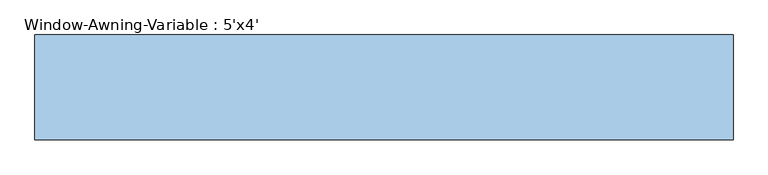
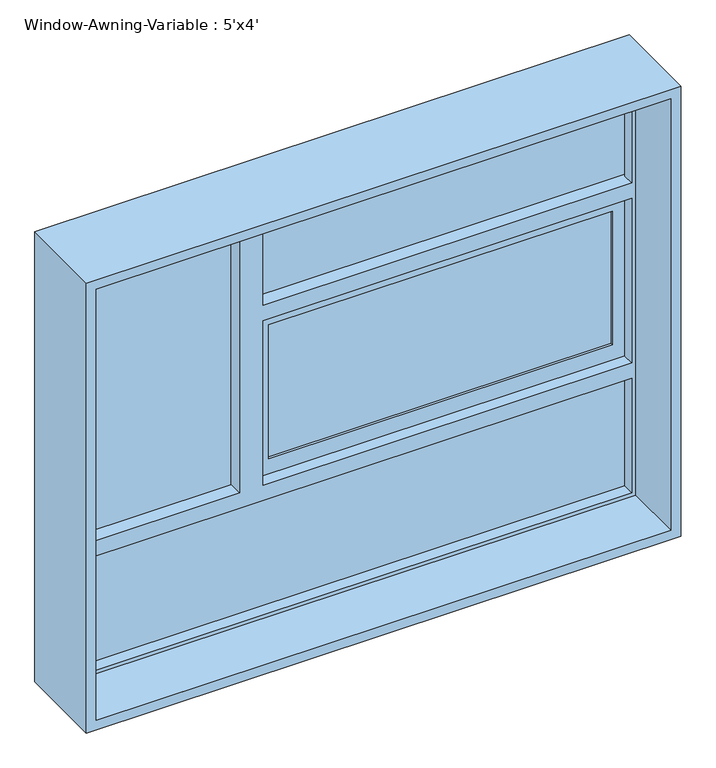
"""IFC4 building model written with IfcOpenShell, lengths in millimetres: window geometry, Window-Awning-Variable : 5'x4'."""

from ifc_helpers import new_model, si_unit, frame, origin, place, context, project, spatial, polyline, outline, extrude, faceted_brep, source, transform, mapped, element, save


def window_awning_variable_5_x4_e7258766(model_context):
    return source(origin(), model_context, "Body", "SolidModel", [
        extrude(outline(polyline([(694.7296875, 98.425), (694.7296875, 92.075), (-186.7296875, 92.075), (-186.7296875, 98.425), (694.7296875, 98.425)])), frame((0.0, 0.0, 1342.9654688), z_axis=(0.0, 0.0, 1.0), x_axis=(1.0, 0.0, 0.0)), (0.0, 0.0, 1.0), 362.0690625),
        extrude(outline(polyline([(694.7296875, 85.725), (694.7296875, 79.375), (-186.7296875, 79.375), (-186.7296875, 85.725), (694.7296875, 85.725)])), frame((0.0, 0.0, 1342.9654688), z_axis=(0.0, 0.0, 1.0), x_axis=(1.0, 0.0, 0.0)), (0.0, 0.0, 1.0), 362.0690625),
        extrude(outline(polyline([(-279.4, 98.425), (-279.4, 92.075), (-736.6, 92.075), (-736.6, 98.425), (-279.4, 98.425)])), frame((0.0, 0.0, 1301.0951563), z_axis=(0.0, 0.0, 1.0), x_axis=(1.0, 0.0, 0.0)), (0.0, 0.0, 1.0), 807.1048438),
        extrude(outline(polyline([(-279.4, 85.725), (-279.4, 79.375), (-736.6, 79.375), (-736.6, 85.725), (-279.4, 85.725)])), frame((0.0, 0.0, 1301.0951563), z_axis=(0.0, 0.0, 1.0), x_axis=(1.0, 0.0, 0.0)), (0.0, 0.0, 1.0), 807.1048438),
        extrude(outline(polyline([(736.6, 85.725), (736.6, 79.375), (-228.6, 79.375), (-228.6, 85.725), (736.6, 85.725)])), frame((0.0, 0.0, 1788.7751563), z_axis=(0.0, 0.0, 1.0), x_axis=(1.0, 0.0, 0.0)), (0.0, 0.0, 1.0), 319.4248438),
        extrude(outline(polyline([(736.6, 98.425), (736.6, 92.075), (-228.6, 92.075), (-228.6, 98.425), (736.6, 98.425)])), frame((0.0, 0.0, 1788.7751563), z_axis=(0.0, 0.0, 1.0), x_axis=(1.0, 0.0, 0.0)), (0.0, 0.0, 1.0), 319.4248438),
        extrude(outline(polyline([(736.6, 98.425), (736.6, 92.075), (-736.6, 92.075), (-736.6, 98.425), (736.6, 98.425)])), frame((0.0, 0.0, 939.8), z_axis=(0.0, 0.0, 1.0), x_axis=(1.0, 0.0, 0.0)), (0.0, 0.0, 1.0), 319.4248438),
        extrude(outline(polyline([(736.6, 85.725), (736.6, 79.375), (-736.6, 79.375), (-736.6, 85.725), (736.6, 85.725)])), frame((0.0, 0.0, 939.8), z_axis=(0.0, 0.0, 1.0), x_axis=(1.0, 0.0, 0.0)), (0.0, 0.0, 1.0), 319.4248438),
        faceted_brep([(-736.6, 73.025, 2108.2), (-736.6, 114.3, 2108.2), (736.6, 114.3, 2108.2), (736.6, 73.025, 2108.2), (-228.6, 73.025, 2108.2), (-228.6, 111.125, 2108.2), (-279.4, 111.125, 2108.2), (-279.4, 73.025, 2108.2), (-726.4796875, 42.06875, 2098.0796875), (-726.4796875, 73.025, 2098.0796875), (-279.4, 73.025, 2098.0796875), (-279.4, 42.06875, 2098.0796875), (726.4796875, 73.025, 2098.0796875), (726.4796875, 42.06875, 2098.0796875), (-218.4796875, 42.06875, 2098.0796875), (-218.4796875, 73.025, 2098.0796875), (-736.6, -114.3, 2108.2), (-736.6, 42.06875, 2108.2), (736.6, 42.06875, 2108.2), (736.6, -114.3, 2108.2), (-762.0, 114.3, 2133.6), (-762.0, -114.3, 2133.6), (762.0, -114.3, 2133.6), (762.0, 114.3, 2133.6), (736.6, 114.3, 939.8), (736.6, 73.025, 939.8), (736.6, 73.025, 1259.2248438), (736.6, 111.125, 1259.2248438), (736.6, 111.125, 1301.0951563), (736.6, 73.025, 1301.0951563), (736.6, 73.025, 1746.9048438), (736.6, 111.125, 1746.9048438), (736.6, 111.125, 1788.7751563), (736.6, 73.025, 1788.7751563), (726.4796875, 73.025, 1788.7751563), (726.4796875, 42.06875, 1788.7751563), (726.4796875, 73.025, 949.9203125), (726.4796875, 42.06875, 949.9203125), (726.4796875, 42.06875, 1259.2248438), (726.4796875, 73.025, 1259.2248438), (726.4796875, 73.025, 1301.0951563), (726.4796875, 42.06875, 1301.0951563), (726.4796875, 42.06875, 1746.9048438), (726.4796875, 73.025, 1746.9048438), (736.6, 42.06875, 939.8), (736.6, -114.3, 939.8), (762.0, -114.3, 914.4), (762.0, 114.3, 914.4), (-736.6, 114.3, 939.8), (-736.6, 73.025, 939.8), (-726.4796875, 73.025, 949.9203125), (-726.4796875, 42.06875, 949.9203125), (-736.6, 42.06875, 939.8), (-736.6, -114.3, 939.8), (-762.0, -114.3, 914.4), (-762.0, 114.3, 914.4), (-736.6, 73.025, 1301.0951563), (-736.6, 111.125, 1301.0951563), (-736.6, 111.125, 1259.2248438), (-736.6, 73.025, 1259.2248438), (-218.4796875, 73.025, 1788.7751563), (-228.6, 73.025, 1788.7751563), (-726.4796875, 73.025, 1259.2248438), (-726.4796875, 73.025, 1301.0951563), (-218.4796875, 73.025, 1301.0951563), (-228.6, 73.025, 1301.0951563), (-228.6, 73.025, 1746.9048438), (-218.4796875, 73.025, 1746.9048438), (-726.4796875, 42.06875, 1301.0951563), (-726.4796875, 42.06875, 1259.2248438), (-218.4796875, 42.06875, 1788.7751563), (-279.4, 42.06875, 1301.0951563), (-218.4796875, 42.06875, 1301.0951563), (-218.4796875, 42.06875, 1746.9048438), (-279.4, 111.125, 1301.0951563), (-228.6, 111.125, 1788.7751563), (-228.6, 111.125, 1746.9048438), (-228.6, 111.125, 1301.0951563)], [[[0, 1, 2, 3, 4, 5, 6, 7]], [[8, 9, 10, 11]], [[12, 13, 14, 15]], [[16, 17, 18, 19]], [[20, 21, 22, 23]], [[3, 2, 24, 25, 26, 27, 28, 29, 30, 31, 32, 33]], [[13, 12, 34, 35]], [[36, 37, 38, 39]], [[40, 41, 42, 43]], [[19, 18, 44, 45]], [[23, 22, 46, 47]], [[25, 24, 48, 49]], [[37, 36, 50, 51]], [[45, 44, 52, 53]], [[47, 46, 54, 55]], [[1, 0, 56, 57, 58, 59, 49, 48]], [[12, 15, 60, 61, 4, 3, 33, 34]], [[25, 49, 59, 62, 50, 36, 39, 26]], [[56, 0, 7, 10, 9, 63]], [[29, 40, 43, 30]], [[64, 65, 66, 67]], [[9, 8, 68, 63]], [[51, 50, 62, 69]], [[52, 44, 18, 17], [14, 13, 35, 70], [37, 51, 69, 38], [68, 8, 11, 71], [72, 73, 42, 41]], [[17, 16, 53, 52]], [[22, 21, 54, 46], [16, 19, 45, 53]], [[21, 20, 55, 54]], [[20, 23, 47, 55], [2, 1, 48, 24]], [[58, 27, 26, 39, 38, 69, 62, 59]], [[27, 58, 57, 74, 6, 5, 75, 32, 31, 76, 77, 28]], [[29, 28, 77, 65, 64, 72, 41, 40]], [[57, 56, 63, 68, 71, 74]], [[6, 74, 71, 11, 10, 7]], [[15, 14, 70, 60]], [[72, 64, 67, 73]], [[5, 4, 61, 75]], [[65, 77, 76, 66]], [[76, 31, 30, 43, 42, 73, 67, 66]], [[32, 75, 61, 60, 70, 35, 34, 33]]]),
        extrude(outline(polyline([(1301.0951563, -228.6), (1301.0951563, 736.6), (1746.9048438, 736.6), (1746.9048438, -228.6), (1301.0951563, -228.6)]), holes=[polyline([(1342.9654688, -186.7296875), (1705.0345313, -186.7296875), (1705.0345313, 694.7296875), (1342.9654688, 694.7296875), (1342.9654688, -186.7296875)])]), frame((0.0, 73.025, 0.0), z_axis=(0.0, 1.0, 0.0), x_axis=(0.0, 0.0, 1.0)), (0.0, 0.0, 1.0), 31.75),
    ])


if __name__ == "__main__":
    model = new_model("IFC4")
    model_context = context("Model", 3, world=origin())
    ifc_project = project(units=[si_unit("LENGTHUNIT", "METRE", prefix="MILLI")], contexts=[model_context])
    site = spatial("IfcSite", under=ifc_project)
    building = spatial("IfcBuilding", under=site)
    placement = place(None, origin())
    window_awning_variable_5_x4_shape = window_awning_variable_5_x4_e7258766(model_context)
    element("IfcWindow", 1, ObjectType="Window-Awning-Variable : 5'x4'", at=placement, inside=building, context=model_context, shape_type="MappedRepresentation", body=[
        mapped(window_awning_variable_5_x4_shape, transform((0.0, 0.0, 0.0), x_axis=(1.0, 0.0, 0.0), y_axis=(0.0, 1.0, 0.0), z_axis=(0.0, 0.0, 1.0))),
    ])
    save(model, "model.ifc")

# Revit data of these elements
# Type "Window-Awning-Variable : 5'x4'"
#   Type Mark = "23"
#   Fire Rating = "0.5h"
#   Assembly Code = "B2020100"
#   Analytic Construction = "Double glazing - domestic"
#   Window Inset [instance default] = 0' - 0 5/8"
#   Wall Thickness [instance default] = 0' - 6"
#   Visual Light Transmittance = 0.81
#   Transom Height Ratio = 0.3
#   Transom Height = 1' - 2.4"
#   Thermal Resistance (R) = 1.8146 (h·ft²·°F)/BTU
#   Solar Heat Gain Coefficient = 0.76
#   Rough Width = 5' - 0 1/2"
#   Rough Height = 4' - 0 1/2"
#   Opening Window Width = 3' - 4"
#   Opening Window Height = 1' - 7.2"
#   Heat Transfer Coefficient (U) = 0.5511 BTU/(h·ft²·°F)
#   Height = 4' - 0"
#   Frame Gap 3 [instance default] = 0' - 1 83/128"
#   Frame Gap 2 [instance default] = 0' - 0 5/8"
#   Frame Gap 1 = 0' - 1 51/128"
#   Fixed Window Width = 1' - 8"
#   Default Sill Height = 3' - 0"
#   Width = 5' - 0"
#   Frame Material = Metal - Aluminum
#   Glass Panel Material = Glass
#   Wall Closure = (empty or 0)
# Element 1 (IfcWindow, "Window-Awning-Variable : 5'x4'")
#   Wall Thickness = 0' - 9"
#   Materials on its faces: "Glass", "Metal - Aluminum"
# Materials
#   "Metal - Aluminum": class "Metal", colour RGB 247 247 247, transparency 0
#   "Glass": class "Glass", colour RGB 0 128 192, transparency 0.75, Description = "Soda Lime Glass", Cost = 0
